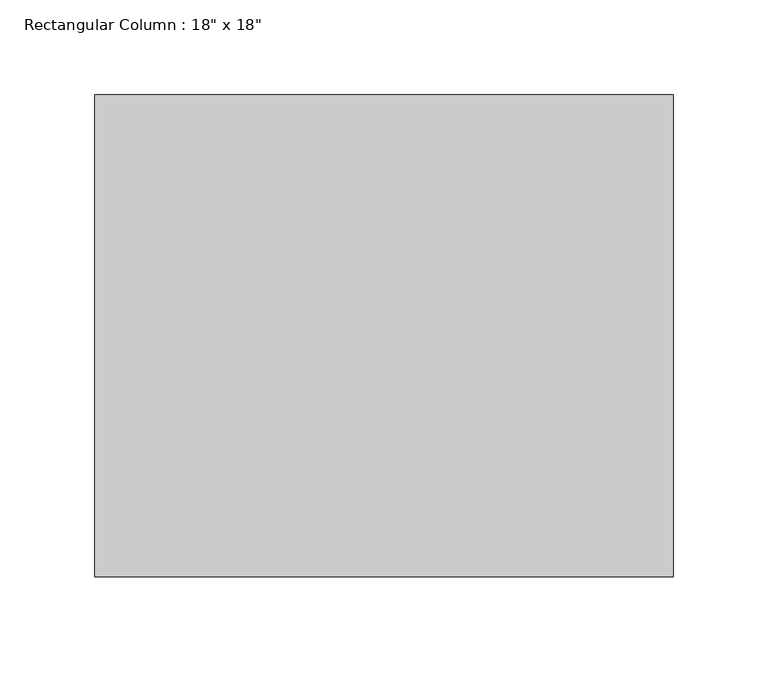
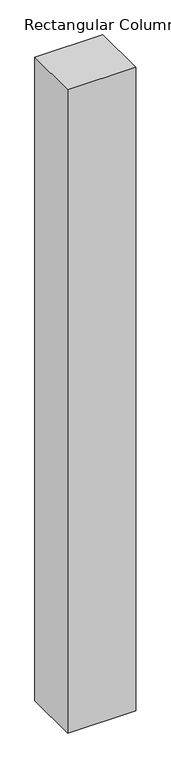
"""IFC4 building model written with IfcOpenShell, lengths in millimetres: column geometry."""

from ifc_helpers import new_model, si_unit, origin, origin_with_axes, place, context, project, spatial, polyline, outline, extrude, source, transform, mapped, element, save


def column_263bc08f(model_context):
    return source(origin(), model_context, "Body", "SweptSolid", [
        extrude(outline(polyline([(152.4, 127.0), (152.4, -127.0), (-152.4, -127.0), (-152.4, 127.0), (152.4, 127.0)])), origin_with_axes(), (0.0, 0.0, 1.0), 3048.0),
    ])


if __name__ == "__main__":
    model = new_model("IFC4")
    model_context = context("Model", 3, world=origin())
    ifc_project = project(units=[si_unit("LENGTHUNIT", "METRE", prefix="MILLI")], contexts=[model_context])
    site = spatial("IfcSite", under=ifc_project)
    building = spatial("IfcBuilding", under=site)
    placement = place(None, origin())
    column_shape = column_263bc08f(model_context)
    element("IfcColumn", 1, ObjectType="Rectangular Column : 18\" x 18\"", at=placement, inside=building, context=model_context, shape_type="MappedRepresentation", body=[
        mapped(column_shape, transform((0.0, 0.0, 0.0), x_axis=(1.0, 0.0, 0.0), y_axis=(0.0, 1.0, 0.0), z_axis=(0.0, 0.0, 1.0))),
    ])
    save(model, "model.ifc")

# Revit data of these elements
# Type "Rectangular Column : 18\" x 18\""
#   Assembly Code = "B1010200"
#   Depth = 0' - 10"
#   Offset Base = 0' - 0"
#   Offset Top = 0' - 0"
#   Width = 1' - 0"
#   Material = Rigid insulation
# Element 1 (IfcColumn, "Rectangular Column : 18\" x 18\"")
#   Materials on its faces: "Rigid insulation"
# Materials
#   "Rigid insulation": class "Generic", colour RGB 127 127 127, transparency 0, Description = "Rigid foam insulation board", Cost = 0
